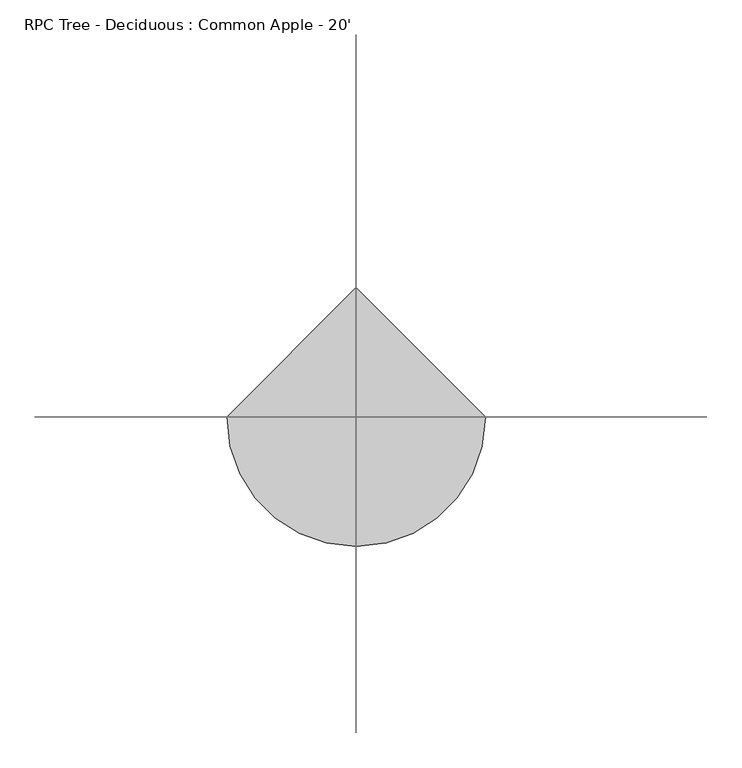
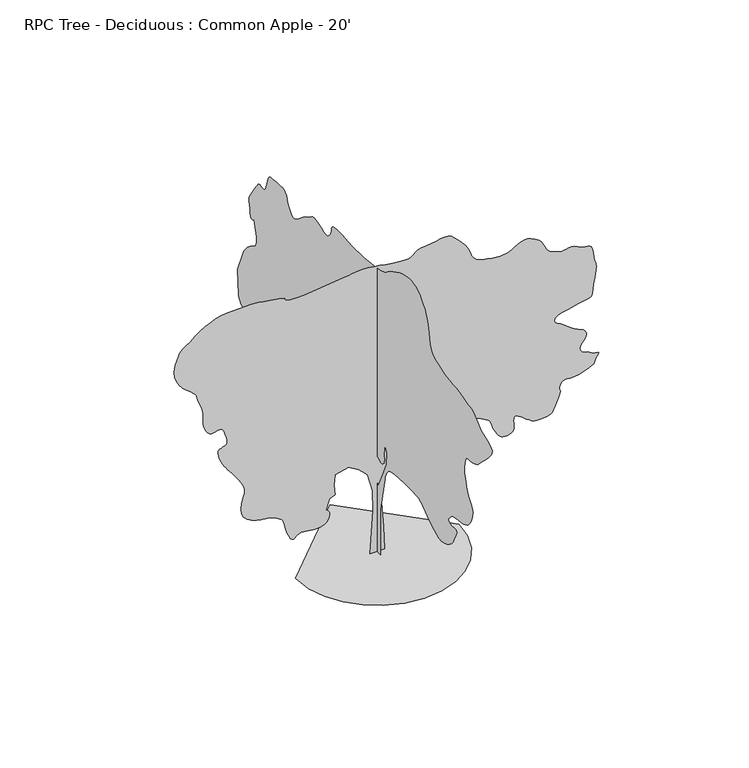
"""IFC4 building model written with IfcOpenShell, lengths in millimetres: geographic element geometry, RPC Tree - Deciduous : Common Apple - 20'."""

from ifc_helpers import new_model, si_unit, origin, place, context, project, spatial, triangles, source, transform, mapped, element, save


def rpc_tree_deciduous_common_apple_20_2cf08d23(model_context):
    return source(origin(), model_context, "Body", "Tessellation", [
        triangles([(-6.61e-05, -106.7031981, 0.0075972), (-6.25e-05, 141.1357166, 0.0075898), (-4.92e-05, 101.4814601, 465.9455781), (-3.19e-05, 131.2220957, 1031.0173004), (-1.83e-05, 230.3576144, 1437.4734501), (-8.7e-06, 398.8869896, 1675.3980263), (-1.1e-06, 587.2459139, 1834.016106), (2.7e-06, 765.6887283, 1873.6680462), (3.6e-06, 963.961219, 1804.2751888), (1.5e-06, 1023.4430534, 1705.1389435), (-4.1e-06, 904.4794573, 1576.2617809), (-8.5e-06, 944.1340136, 1407.7326782), (-1.46e-05, 1172.144878, 1090.4990622), (-1.49e-05, 1568.687534, 882.3128597), (-8.7e-06, 2143.6727863, 803.006436), (7.7e-06, 2490.6473923, 1179.7191977), (2.57e-05, 2847.5453751, 1606.0026981), (3.25e-05, 3402.6882339, 1556.4345028), (3.9e-05, 3600.9610153, 1675.3980263), (4.6e-05, 3591.0549339, 1913.3226025), (4.57e-05, 3412.6196045, 1992.6315697), (5.03e-05, 3283.7399712, 2210.7288677), (5.51e-05, 3591.0549339, 2220.6425068), (6.07e-05, 4205.6845688, 2101.6814541), (6.29e-05, 4275.3567696, 2137.8384041), (6.49e-05, 4342.3114037, 2174.2544952), (6.7e-05, 4403.9061905, 2211.1911942), (6.89e-05, 4457.4241447, 2248.9101128), (7.07e-05, 4500.1976967, 2287.6680668), (7.23e-05, 4529.5348595, 2327.7263775), (7.37e-05, 4542.7427742, 2369.3469475), (8.93e-05, 4572.4863075, 2874.9268433), (9.94e-05, 4403.9570595, 3301.215358), (0.0001002, 4386.5834106, 3334.8449913), (0.000101, 4360.9041641, 3374.6975006), (0.0001018, 4328.265168, 3418.5378479), (0.0001026, 4290.0887192, 3464.105706), (0.0001033, 4247.7471176, 3509.1651649), (0.0001039, 4202.636499, 3551.4561882), (0.0001043, 4156.1291634, 3588.718158), (0.0001045, 4111.323468, 3617.9027138), (0.0001046, 4070.8611122, 3640.1530998), (0.0001046, 4035.4281006, 3659.4571541), (0.0001048, 4005.7101471, 3679.8024239), (0.0001052, 3982.4182549, 3705.2026176), (0.000106, 3966.2384285, 3739.5941231), (0.0001073, 3957.8566727, 3786.9906487), (0.0001089, 3956.7898773, 3842.7945099), (0.0001107, 3961.4378494, 3899.6395866), (0.0001126, 3970.8614021, 3957.3738533), (0.0001145, 3984.0948967, 4015.7685448), (0.0001165, 4000.1982742, 4074.6966339), (0.0001185, 4018.2070587, 4133.9802246), (0.0001206, 4037.1553207, 4193.4417114), (0.0001203, 4062.5299347, 4172.9947037), (0.0001202, 4087.2188347, 4157.4244331), (0.0001204, 4110.5107269, 4151.5570587), (0.000121, 4131.7196068, 4160.2693176), (0.0001221, 4150.160051, 4188.3870781), (0.0001239, 4165.1460548, 4240.787368), (0.0001265, 4175.9410355, 4322.3213448), (0.000129, 4186.6092796, 4402.5600517), (0.0001308, 4198.1408432, 4455.5698975), (0.000132, 4205.3543564, 4492.9588943), (0.000133, 4202.9922913, 4526.3597626), (0.0001339, 4185.923275, 4567.406385), (0.0001352, 4148.8900703, 4627.7059021), (0.000137, 4086.736306, 4718.8666168), (0.0001389, 4019.8834099, 4816.9867905), (0.0001404, 3969.4896835, 4892.043837), (0.0001414, 3931.4405525, 4946.4759796), (0.0001421, 3901.5194138, 4982.6714447), (0.0001423, 3875.5858223, 5003.1184525), (0.0001421, 3849.5002052, 5010.2046478), (0.0001416, 3819.0709579, 5006.343837), (0.0001408, 3787.3208611, 4996.7176804), (0.0001401, 3759.4062859, 4987.6240494), (0.0001396, 3734.2601463, 4983.2045517), (0.0001394, 3710.841227, 4987.6240494), (0.0001396, 3688.1338921, 5005.0485672), (0.0001402, 3665.0704742, 5039.6435486), (0.0001416, 3640.6103394, 5095.574437), (0.0001432, 3619.2235634, 5160.9030075), (0.0001447, 3603.043737, 5219.9581238), (0.000146, 3587.5496246, 5271.4183548), (0.000147, 3568.2455704, 5313.8366959), (0.0001475, 3540.6103386, 5345.8661362), (0.0001475, 3500.1482735, 5366.109668), (0.0001469, 3442.3378487, 5373.1458664), (0.0001459, 3372.4368828, 5376.2445145), (0.0001451, 3300.6055115, 5383.3312912), (0.0001442, 3229.8412262, 5391.1034912), (0.0001434, 3163.0391991, 5396.2851517), (0.0001425, 3103.1713417, 5395.5485687), (0.0001414, 3053.2095657, 5385.642778), (0.0001402, 3016.0746231, 5363.2394943), (0.0001391, 2991.8429626, 5337.2044556), (0.0001382, 2976.4758774, 5316.3510773), (0.0001375, 2966.6462448, 5297.4283951), (0.0001368, 2959.0769394, 5277.1081238), (0.0001359, 2950.4664185, 5252.1148819), (0.0001348, 2937.5122673, 5219.1198029), (0.0001331, 2916.9382324, 5174.873085), (0.0001313, 2890.1666107, 5126.1051315), (0.0001296, 2860.6265533, 5083.2042618), (0.000128, 2827.9619774, 5048.4569641), (0.0001268, 2791.8432518, 5024.124147), (0.0001258, 2751.8890045, 5012.4399765), (0.0001253, 2707.794603, 5015.6909409), (0.0001252, 2659.1789658, 5036.0873703), (0.0001254, 2610.791803, 5068.0662323), (0.0001258, 2565.8846603, 5103.6768494), (0.0001263, 2521.8332794, 5141.7006912), (0.0001267, 2476.0523529, 5180.9436447), (0.0001272, 2425.9356445, 5220.212178), (0.0001274, 2368.8821503, 5258.2360199), (0.0001275, 2302.2908661, 5293.846637), (0.0001276, 2240.2945049, 5328.4671982), (0.0001279, 2193.5584042, 5362.0459625), (0.0001282, 2154.2798424, 5391.129071), (0.0001282, 2114.6558075, 5412.2365036), (0.0001278, 2066.8783459, 5421.8882401), (0.0001267, 2003.1496777, 5416.6304214), (0.0001247, 1915.6618492, 5392.9830276), (0.0001224, 1826.1497257, 5361.2837997), (0.0001207, 1757.9710384, 5335.9853439), (0.0001194, 1705.7434124, 5319.8816757), (0.0001187, 1664.0950825, 5315.7418121), (0.0001184, 1627.6484699, 5326.358606), (0.0001187, 1591.0293388, 5354.4766571), (0.0001195, 1548.8602558, 5402.8893997), (0.0001207, 1514.8419834, 5459.7853455), (0.000122, 1498.8602554, 5510.7630478), (0.0001232, 1489.8128426, 5554.806871), (0.0001241, 1476.6047825, 5590.874437), (0.0001244, 1448.1338459, 5617.9256927), (0.0001241, 1393.3079773, 5634.9182602), (0.0001229, 1301.0220406, 5640.8109238), (0.0001214, 1201.3955635, 5639.6935501), (0.0001202, 1126.7398006, 5636.6454803), (0.0001192, 1069.2519579, 5632.2259827), (0.0001184, 1021.1290958, 5626.9425842), (0.0001175, 974.5682751, 5621.3039749), (0.0001165, 921.7642307, 5615.8426804), (0.0001154, 854.9113346, 5611.0679718), (0.0001143, 784.7082069, 5608.019902), (0.0001133, 723.0014357, 5607.2071609), (0.0001125, 663.7228592, 5608.4768509), (0.0001116, 600.8019178, 5611.6516571), (0.0001107, 528.1680156, 5616.5792633), (0.0001096, 439.7556433, 5623.0567749), (0.0001082, 329.4941322, 5630.9051331), (0.0001067, 206.9466705, 5641.7254028), (0.0001053, 88.3885184, 5656.6861176), (0.0001042, -22.1921751, 5675.1262711), (0.0001034, -120.8075788, 5696.3354416), (0.0001029, -203.4686488, 5719.6276245), (0.0001027, -266.1871316, 5744.3162338), (0.0001028, -304.9729546, 5769.6908478), (0.0001032, -347.9523442, 5804.4381454), (0.0001036, -420.583703, 5853.4089935), (0.0001039, -514.8939712, 5910.1532043), (0.000104, -622.9024584, 5968.31884), (0.0001039, -736.6335978, 6021.4301331), (0.0001035, -848.1092062, 6063.1118912), (0.0001027, -949.3562239, 6086.9371811), (0.0001016, -1039.2697763, 6095.8017563), (0.0001004, -1122.4243664, 6096.0046509), (9.9e-05, -1199.3330441, 6086.1494385), (9.73e-05, -1270.5191059, 6064.8391113), (9.53e-05, -1336.5033051, 6030.7016602), (9.29e-05, -1397.8062492, 5982.3650757), (9.01e-05, -1454.9462208, 5918.407933), (8.77e-05, -1502.3755932, 5861.1056168), (8.62e-05, -1536.9730453, 5825.4944183), (8.5e-05, -1562.8963177, 5799.256485), (8.38e-05, -1584.313615, 5770.0716385), (8.22e-05, -1605.3828232, 5725.6220261), (7.96e-05, -1630.2698215, 5653.5874695), (7.58e-05, -1663.1323505, 5541.6751144), (7.16e-05, -1693.8258259, 5415.6147858), (6.81e-05, -1715.6747829, 5307.5626602), (6.5e-05, -1738.0446384, 5214.9799393), (6.21e-05, -1770.3000824, 5135.1981812), (5.93e-05, -1821.8062408, 5065.6530075), (5.62e-05, -1901.9230076, 5003.7532974), (5.28e-05, -2020.0178341, 4946.8823502), (4.95e-05, -2152.913356, 4902.7117905), (4.69e-05, -2273.494804, 4876.3974083), (4.48e-05, -2385.2295536, 4861.5384315), (4.29e-05, -2491.5921021, 4851.7340881), (4.1e-05, -2596.0345642, 4840.5071571), (3.89e-05, -2702.0542557, 4821.482737), (3.62e-05, -2813.1030006, 4788.2594742), (3.39e-05, -2912.3155495, 4758.5159409), (3.24e-05, -2986.585144, 4746.9843773), (3.14e-05, -3044.8780975, 4742.742485), (3.04e-05, -3096.2371719, 4734.8432579), (2.89e-05, -3149.6786774, 4712.3896866), (2.66e-05, -3214.2200867, 4664.4344742), (2.28e-05, -3298.878582, 4580.0809021), (1.85e-05, -3408.6320572, 4492.8062874), (1.5e-05, -3530.0185432, 4434.3354378), (1.2e-05, -3644.3188339, 4390.95233), (9.4e-06, -3732.7616913, 4348.9659393), (7.2e-06, -3776.6273277, 4294.6608238), (5.1e-06, -3757.196537, 4214.3459587), (3e-06, -3655.7486595, 4094.3056114), (1.1e-06, -3529.027906, 3968.7786804), (-3e-07, -3439.3912262, 3876.7287758), (-1.3e-06, -3376.6531952, 3811.5525215), (-1.9e-06, -3330.5522301, 3766.670668), (-2.3e-06, -3290.852037, 3735.479258), (-2.3e-06, -3247.3671913, 3711.4002045), (-2.2e-06, -3189.8108208, 3687.854258), (-1.7e-06, -3124.3802216, 3671.1919029), (-1e-06, -3064.487075, 3666.3404549), (-2e-07, -3010.8420937, 3664.4356293), (2e-07, -2964.1568619, 3656.6378494), (2e-07, -2925.0662247, 3634.0825401), (-8e-07, -2894.3070557, 3587.9559952), (-2.8e-06, -2872.5897766, 3509.3939301), (-5.1e-06, -2860.8041588, 3423.8465355), (-7.1e-06, -2858.3659355, 3357.9081184), (-8.8e-06, -2863.7507813, 3304.4410332), (-1.04e-05, -2875.358503, 3256.3335045), (-1.21e-05, -2891.6653564, 3206.498465), (-1.41e-05, -2911.070858, 3147.8244301), (-1.67e-05, -2932.0768433, 3073.199334), (-1.95e-05, -2961.2613991, 2993.8242371), (-2.22e-05, -3001.7234642, 2923.6186386), (-2.47e-05, -3046.5291595, 2859.6612053), (-2.72e-05, -3088.7187355, 2798.9806068), (-2.95e-05, -3121.3830208, 2738.6555099), (-3.16e-05, -3137.5628471, 2675.7398735), (-3.35e-05, -3130.349334, 2607.2612045), (-3.52e-05, -3109.3942177, 2540.281572), (-3.66e-05, -3087.7280983, 2482.819091), (-3.77e-05, -3063.4964378, 2433.5098915), (-3.85e-05, -3034.7182526, 2390.964814), (-3.91e-05, -2999.5645844, 2353.7970245), (-3.94e-05, -2956.0544495, 2320.6169277), (-3.96e-05, -2902.3333099, 2290.0378349), (-3.93e-05, -2836.3948929, 2266.2507694), (-3.86e-05, -2760.9314758, 2251.4832115), (-3.77e-05, -2680.9721123, 2241.3942924), (-3.68e-05, -2601.4955681, 2231.6559334), (-3.61e-05, -2527.6041481, 2217.9272655), (-3.58e-05, -2464.279525, 2195.8749779), (-3.62e-05, -2416.56049, 2161.1632885), (-3.68e-05, -2383.2356346, 2123.2410393), (-3.73e-05, -2359.9691769, 2093.2995529), (-3.79e-05, -2347.1065899, 2069.598674), (-3.84e-05, -2344.9984337, 2050.4090023), (-3.9e-05, -2353.9875652, 2033.9929985), (-3.98e-05, -2374.4217831, 2018.6158848), (-4.07e-05, -2406.646851, 2002.5452087), (-4.16e-05, -2449.8269188, 1993.9041664), (-4.23e-05, -2498.3841293, 1996.5330757), (-4.28e-05, -2545.5646797, 2002.2862129), (-4.34e-05, -2584.5791588, 2003.0075352), (-4.41e-05, -2608.6837921, 1990.5513187), (-4.52e-05, -2611.0967262, 1956.7642822), (-4.66e-05, -2585.0869766, 1893.4953243), (-4.83e-05, -2549.9080193, 1821.1814243), (-4.96e-05, -2524.6272949, 1762.91376), (-5.07e-05, -2502.1126808, 1714.5318295), (-5.16e-05, -2475.2625755, 1671.8725147), (-5.23e-05, -2436.9668026, 1630.7726978), (-5.27e-05, -2380.1140228, 1587.0720222), (-5.3e-05, -2297.5969666, 1536.6072247), (-5.28e-05, -2203.8378639, 1496.8968578), (-5.19e-05, -2116.842738, 1484.7582092), (-5.03e-05, -2034.8743401, 1494.9892708), (-4.83e-05, -1956.2028339, 1522.3883251), (-4.6e-05, -1879.090971, 1561.7532188), (-4.35e-05, -1801.803828, 1607.8822346), (-4.09e-05, -1722.6115688, 1655.5707481), (-3.83e-05, -1647.9584221, 1703.6352562), (-3.59e-05, -1583.013113, 1752.3931812), (-3.37e-05, -1524.1383636, 1798.8980461), (-3.16e-05, -1467.6919544, 1840.2010483), (-2.97e-05, -1410.0313751, 1873.3506237), (-2.82e-05, -1347.5167316, 1895.4053822), (-2.69e-05, -1276.503479, 1903.4089634), (-2.54e-05, -1177.6846561, 1904.2776604), (-2.33e-05, -1044.3574018, 1905.4916851), (-2.11e-05, -891.7820492, 1904.9710773), (-1.89e-05, -735.2163151, 1900.6352955), (-1.7e-05, -589.9230761, 1890.4040886), (-1.58e-05, -471.1627742, 1872.1948803), (-1.55e-05, -394.1956335, 1843.9297451), (-1.6e-05, -348.7041879, 1805.3140789), (-1.68e-05, -313.0958962, 1758.377409), (-1.8e-05, -285.7248199, 1704.5039532), (-1.95e-05, -264.9450744, 1645.0805454), (-2.11e-05, -249.1058704, 1581.494165), (-2.29e-05, -236.5620685, 1515.1341167), (-2.48e-05, -225.6659676, 1447.3870892), (-3.91e-05, -116.6168281, 912.0537769), (-2.05e-05, -27.3946828, 1318.5099266), (-1.32e-05, -176.0980811, 1635.74347), (-6.6e-06, -304.975498, 1923.2362415), (2e-07, -324.8002327, 2161.1632885), (4.8e-06, -255.4073572, 2280.1241959), (-4e-07, -225.6657133, 2091.767815), (-1.7e-06, -231.7353101, 2049.4539734), (-3e-06, -235.984215, 2008.1814926), (-4.2e-06, -236.5910275, 1968.9892628), (-5.2e-06, -231.7353101, 1932.9186447), (-6e-06, -219.5961346, 1901.0111446), (-6.5e-06, -198.3530817, 1874.3056526), (-6.6e-06, -166.1844602, 1853.8433842), (-6.2e-06, -129.2182845, 1848.5829494), (-5.3e-06, -95.0268123, 1860.3152275), (-4.3e-06, -63.9562343, 1879.3348515), (-3.4e-06, -36.354542, 1895.9235191), (-2.9e-06, -12.5678035, 1900.3761543), (-3.1e-06, 7.0569383, 1882.9772163), (-4.4e-06, 22.1729471, 1834.016106), (-6.1e-06, 32.8958209, 1768.9260384), (-7.8e-06, 39.9768386, 1709.0403042), (-9.4e-06, 44.0233167, 1653.4904972), (-1.1e-05, 45.6418044, 1601.4077751), (-1.24e-05, 45.4396183, 1551.9260571), (-1.39e-05, 44.0233167, 1504.1789715), (-1.53e-05, 41.9999482, 1457.3007282), (139.590126, 0.0003305, 0.0), (-135.4471285, 0.0003387, 0.0), (-74.3278259, 0.000241, 845.4879272), (-84.5142454, 0.0002472, 1242.76455), (-186.3807747, 0.0002013, 1599.294532), (-339.1791879, 0.0002082, 1752.0933449), (-542.9102117, 0.000216, 1874.3335579), (-797.5758808, 0.0002227, 1813.2134514), (-817.9492012, 0.0002203, 1609.4824276), (-797.5758808, 0.0002168, 1415.9368286), (-899.4426281, 0.0002191, 1365.0021469), (-970.7481594, 0.0002183, 1171.4565479), (-951.3247084, 0.0002718, 1158.1240768), (-933.2373676, 0.000271, 1143.3616058), (-917.8246456, 0.0002703, 1125.7517796), (-906.4200365, 0.0002696, 1103.8645981), (-900.3621214, 0.000269, 1076.2750757), (-900.9870106, 0.0002686, 1041.555756), (-909.6280529, 0.0002682, 998.2868128), (-928.5764603, 0.0002681, 955.1042742), (-957.6798437, 0.0002684, 921.0098436), (-994.6267164, 0.0002692, 895.1144766), (-1037.0955631, 0.0002701, 876.5217161), (-1082.7698101, 0.0002713, 864.3449158), (-1129.3382612, 0.0002726, 857.6926329), (-1174.4791832, 0.0002739, 855.6733521), (-1218.6700905, 0.0002753, 858.4063974), (-1263.5747623, 0.0002767, 865.0586803), (-1308.6573303, 0.0002782, 873.3161705), (-1353.3816353, 0.0002796, 880.857498), (-1397.217041, 0.000281, 885.3710306), (-1439.6273884, 0.0002823, 884.5404854), (-1480.0769543, 0.0002833, 876.0466724), (-1514.854628, 0.0002841, 857.900905), (-1542.5051205, 0.0002846, 834.4084436), (-1565.8782578, 0.000285, 812.6990856), (-1587.8238659, 0.0002854, 799.9000122), (-1611.1970032, 0.0002862, 803.1359339), (-1638.8473503, 0.0002874, 829.5392641), (-1673.6225533, 0.000235, 886.2346407), (-1706.6171963, 0.0002371, 959.4984827), (-1729.2790398, 0.0002388, 1029.5593225), (-1744.988982, 0.0002402, 1094.4487484), (-1757.1353336, 0.0002415, 1152.2135365), (-1769.1037891, 0.0002426, 1200.8900711), (-1784.2803337, 0.0002436, 1238.5177162), (-1806.0481911, 0.0002446, 1263.1378704), (-1833.1626698, 0.0002457, 1282.7670502), (-1863.3073414, 0.0002469, 1305.4288937), (-1898.2629112, 0.0002483, 1329.1576778), (-1939.8122646, 0.0002499, 1351.9948013), (-1989.7334908, 0.0002517, 1371.9820988), (-2049.8147072, 0.0002537, 1387.1586433), (-2121.8338577, 0.000256, 1395.5635082), (-2205.4938675, 0.0002044, 1404.6210949), (-2294.67854, 0.0002073, 1424.3695988), (-2382.4381542, 0.0002104, 1456.7724174), (-2461.8232796, 0.0002135, 1503.7853909), (-2525.8821602, 0.0002163, 1567.3691551), (-2567.6627495, 0.0002188, 1649.4849277), (-2580.2355286, 0.0002207, 1752.0933449), (-2568.9835991, 0.0002218, 1851.4048702), (-2548.8159348, 0.0002224, 1927.9097935), (-2527.0379036, 0.0002227, 1989.979842), (-2510.9723145, 0.0001688, 2045.9893593), (-2507.9117455, 0.0001695, 2104.3180664), (-2525.1659248, 0.0001711, 2173.3375454), (-2570.0503944, 0.0001737, 2261.4222851), (-2629.7912247, 0.0001769, 2355.7756828), (-2686.3316689, 0.0001798, 2438.7243988), (-2738.9604332, 0.0001825, 2511.3356644), (-2786.9665146, 0.0001849, 2574.6730774), (-2829.6130394, 0.0001327, 2629.841803), (-2866.1890045, 0.0001345, 2677.8478844), (-2896.008696, 0.000136, 2719.8086952), (-2924.6092758, 0.0001376, 2767.4084061), (-2955.1652596, 0.0001394, 2827.2762634), (-2983.4100471, 0.0001412, 2893.0114952), (-3005.0764572, 0.0001428, 2958.2389091), (-3015.8461487, 0.000144, 3016.5062828), (-3011.4772293, 0.0001446, 3061.4137161), (-2987.7028084, 0.0001442, 3086.5342758), (-2951.4823448, 0.0001433, 3098.8532913), (-2915.109565, 0.0001425, 3111.5533882), (-2882.1147766, 0.0001417, 3127.4282913), (-2856.0800285, 0.0001413, 3149.3740448), (-2840.5350471, 0.0001413, 3180.2349518), (-2839.0871704, 0.0001418, 3222.8561874), (-2855.2669968, 0.0001432, 3280.0823456), (-2877.0348541, 9.05e-05, 3338.9342766), (-2892.2240433, 9.16e-05, 3385.5177704), (-2904.1875572, 9.25e-05, 3421.2048363), (-2916.3286766, 9.32e-05, 3447.4686401), (-2932.0259743, 9.4e-05, 3465.705899), (-2954.70802, 9.48e-05, 3477.3389099), (-2987.7028084, 9.59e-05, 3483.8161308), (-3026.4123642, 9.7e-05, 3481.8857254), (-3064.2583099, 9.8e-05, 3472.1066711), (-3101.5455688, 9.9e-05, 3461.6419029), (-3138.6805115, 0.0001, 3457.552327), (-3175.9930595, 0.0001013, 3467.026458), (-3213.8137161, 0.0001029, 3497.1763618), (-3252.5488518, 0.0001049, 3555.1138138), (-3281.1747208, 0.0001068, 3626.7419998), (-3293.239682, 0.0001082, 3695.3474052), (-3295.8558014, 0.0001093, 3764.1307068), (-3296.1351448, 0.0001104, 3836.3175797), (-3301.2406471, 5.74e-05, 3915.0575409), (-3318.2840836, 5.93e-05, 4003.6274254), (-3354.4028091, 6.19e-05, 4105.2020393), (-3391.2836975, 6.43e-05, 4197.0231789), (-3411.2481766, 6.59e-05, 4259.8120789), (-3422.2972115, 6.68e-05, 4301.925206), (-3432.4570564, 6.76e-05, 4331.7448975), (-3449.7545471, 6.85e-05, 4357.6276199), (-3482.1650688, 6.99e-05, 4387.9804184), (-3537.7657448, 7.22e-05, 4431.1606316), (-3609.6985634, 2.09e-05, 4488.5646858), (-3681.631382, 2.41e-05, 4556.1285851), (-3747.3157448, 2.72e-05, 4634.0305161), (-3800.5287758, 3.01e-05, 4722.4480843), (-3835.047599, 3.26e-05, 4821.5588951), (-3844.6231773, 3.45e-05, 4931.5152649), (-3822.9823471, 3.57e-05, 5052.5468307), (-3789.555899, -1.8e-05, 5157.9310959), (-3763.7749146, -1.77e-05, 5228.187854), (-3739.5941231, -1.77e-05, 5274.3902664), (-3710.9682541, -1.81e-05, 5307.5882401), (-3671.8270386, -1.88e-05, 5338.8555176), (-3616.1246246, -1.98e-05, 5379.1652664), (-3537.7657448, -2.13e-05, 5439.6429703), (-3445.4364967, -2.3e-05, 5511.6775269), (-3351.6849518, -2.48e-05, 5578.225209), (-3256.3079247, -2.67e-05, 5637.4326416), (-3159.1783882, -2.89e-05, 5687.5726044), (-3060.0675774, -3.12e-05, 5726.8155579), (-2958.8228851, -3.39e-05, 5753.4348633), (-2855.2669968, -3.68e-05, 5765.6015625), (-2376.4970924, -5.09e-05, 5775.7869873), (-2309.7356152, -5.29e-05, 5773.1197083), (-2232.8167637, -5.53e-05, 5765.6521408), (-2147.4320045, -3.8e-06, 5754.1458664), (-2055.2781818, -6.7e-06, 5739.4392059), (-1958.0469074, -9.9e-06, 5722.3449005), (-1857.4273224, -1.32e-05, 5703.6251129), (-1755.1159801, -1.65e-05, 5684.1181641), (-1751.9080364, -1.69e-05, 5664.6617935), (-1742.5530842, -1.75e-05, 5646.3739563), (-1720.9022255, -1.83e-05, 5630.3970245), (-1680.8107773, -1.97e-05, 5617.9001129), (-1616.1270802, -2.18e-05, 5610.0261749), (-1520.7042709, -2.46e-05, 5607.9437439), (-1388.3981026, -2.85e-05, 5612.8201904), (-614.2181774, -5.02e-05, 5704.4890137), (-538.3076946, -5.24e-05, 5711.4996323), (-472.1990845, 1e-07, 5721.8879517), (-409.4762778, -1.6e-06, 5732.8355392), (-343.7232419, -3.5e-06, 5741.4460602), (-268.5264692, -5.7e-06, 5744.8749207), (-177.4707081, -8.5e-06, 5740.3031067), (-64.1414019, -1.21e-05, 5724.8598633), (54.7118994, -1.59e-05, 5704.3111176), (159.4882483, -1.93e-05, 5686.4296509), (252.3260954, -2.23e-05, 5671.4183578), (335.3640864, -2.49e-05, 5659.4039749), (410.7386644, -2.73e-05, 5650.6155579), (480.5886887, -2.95e-05, 5645.205423), (547.0529457, -3.15e-05, 5643.3764648), (603.2428662, -3.3e-05, 5651.8346695), (646.0698669, -3.4e-05, 5673.6531052), (683.3697704, -3.47e-05, 5703.4983765), (722.9887184, -3.54e-05, 5736.0359253), (772.7625698, -3.64e-05, 5765.8806152), (840.5349592, -3.81e-05, 5787.6996323), (934.1441437, -4.07e-05, 5796.1828354), (1035.6832947, -4.37e-05, 5802.989978), (1124.0372766, -4.61e-05, 5818.3826431), (1202.2337391, -4.82e-05, 5834.6642075), (1273.3004768, -5.01e-05, 5844.1636276), (1340.2726971, -5.22e-05, 5839.2360214), (1406.173035, -5.46e-05, 5812.2103455), (1474.0342999, -3.2e-06, 5755.4161377), (1539.0152172, -6.2e-06, 5686.9627579), (1594.7301304, -8.7e-06, 5628.1366974), (1641.8903332, -1.09e-05, 5576.0666199), (1681.2120609, -1.28e-05, 5527.9335114), (1713.4041367, -1.44e-05, 5480.8671982), (1739.182505, -1.59e-05, 5431.9975067), (1759.2587505, -1.73e-05, 5378.5304214), (1777.3156425, -1.87e-05, 5324.8604416), (1798.9361252, -2e-05, 5277.2604401), (1827.6839344, -2.15e-05, 5235.5281036), (1867.1225155, 3.1e-05, 5199.4855362), (1920.8180752, 2.9e-05, 5169.0060013), (1992.3318787, 2.65e-05, 5143.8342819), (2085.229842, 2.34e-05, 5123.844223), (2181.6306438, 2.03e-05, 5109.4171967), (2262.7075264, 1.78e-05, 5100.6799393), (2330.5991673, 1.57e-05, 5097.123761), (2387.4419186, 1.4e-05, 5098.1905563), (2435.3767834, 1.27e-05, 5103.3722168), (2476.5374977, 1.16e-05, 5112.0844757), (2513.0678261, 1.07e-05, 5123.844223), (2552.2195061, 9.8e-06, 5144.4947067), (2599.1840813, 8.9e-06, 5175.4829315), (2653.1336952, 7.8e-06, 5209.6459625), (2713.1032906, 6.4e-06, 5239.9226028), (2778.2795448, 4.8e-06, 5259.1249191), (2847.697982, 2.7e-06, 5260.1661346), (2920.5196999, 2e-07, 5235.9094757), (2984.2992371, -2.2e-06, 5202.1528152), (3030.2478859, -4e-06, 5176.5747253), (3062.9883293, -5.3e-06, 5154.908606), (3087.1947006, -6.3e-06, 5132.9122742), (3107.4893921, -7.3e-06, 5106.2679703), (3128.4697975, -8.5e-06, 5070.73293), (3154.8094688, -1e-05, 5021.9905563), (3182.8510712, 4.27e-05, 4971.0890121), (3208.2256851, 4.13e-05, 4930.3473129), (3234.4639091, 4e-05, 4897.4289734), (3265.1724998, 3.87e-05, 4870.0475052), (3303.9076355, 3.72e-05, 4845.8667137), (3354.2252037, 3.53e-05, 4822.6004013), (3419.6808014, 3.3e-05, 4797.8859215), (3486.0258797, 3.08e-05, 4782.8237595), (3540.0769409, 2.92e-05, 4784.7032959), (3586.9909378, 2.8e-05, 4795.4729874), (3631.9489494, 2.68e-05, 4807.1571579), (3680.1326363, 2.55e-05, 4811.7036827), (3736.6730804, 2.36e-05, 4801.0863075), (3806.7519424, 2.1e-05, 4767.3299377), (3879.2181587, 1.84e-05, 4732.9890106), (3939.9240463, 1.63e-05, 4718.4346664), (3989.5811897, 1.48e-05, 4712.2626595), (4028.9003014, 1.35e-05, 4703.0678719), (4058.6185455, 1.22e-05, 4679.4204781), (4079.3957657, 6.51e-05, 4629.9412308), (4091.9941246, 6.34e-05, 4543.2253029), (4103.8306114, 6.18e-05, 4454.6301292), (4119.4261711, 6.04e-05, 4397.0481789), (4135.0217308, 5.94e-05, 4355.3161331), (4146.8835068, 5.84e-05, 4314.2950905), (4151.2268463, 5.74e-05, 4258.8467308), (4144.3688347, 5.64e-05, 4173.8330246), (4122.550399, 5.51e-05, 4044.0642014), (4100.096537, 0.000108, 3908.7329269), (4088.8698967, 0.0001069, 3812.0603394), (4081.3767494, 0.0001061, 3746.5791618), (4070.1501091, 0.0001058, 3704.7962471), (4047.6965378, 0.0001061, 3679.2184479), (4006.548468, 0.0001071, 3662.4034859), (3939.1874634, 0.0001089, 3646.8079262), (3844.4708611, 0.0001114, 3628.5706673), (3734.0822502, 0.0001144, 3608.1998177), (3619.7822502, 0.0001175, 3584.781189), (3513.3053192, 0.0001202, 3557.4761696), (3426.4373657, 0.0001224, 3525.3449913), (3370.9384277, 0.0001234, 3487.4990456), (3358.5429634, 0.0001231, 3443.0744316), (3371.5224037, 0.0001222, 3405.6092766), (3386.2799332, 0.0001214, 3384.1972115), (3405.8633308, 0.0001207, 3371.1669022), (3433.2700882, 0.0001197, 3358.8478867), (3471.5476936, 0.0001182, 3339.5694122), (3523.7447983, 0.0001162, 3305.6857246), (3592.8327324, 0.0001133, 3249.5260712), (3669.2870773, 0.0001101, 3189.9884262), (3740.381575, 0.0001074, 3147.3671906), (3804.5419029, 0.000105, 3116.150782), (3860.1425789, 0.0001572, 3090.8014572), (3905.55783, 0.0001555, 3065.8332138), (3939.2383324, 0.000154, 3035.6833099), (3959.558313, 0.0001528, 2994.8654526), (3960.2948959, 0.0001521, 2946.884951), (3941.8038734, 0.0001519, 2899.2852402), (3912.2635254, 0.0001521, 2852.3968231), (3879.8530037, 0.0001524, 2806.5752014), (3852.8020386, 0.0001525, 2762.1758766), (3839.2892006, 0.0001523, 2719.554641), (3847.5189308, 0.0001514, 2679.0672867), (3870.582058, 0.0001503, 2647.1645828), (3896.1598572, 0.0001492, 2627.2256836), (3924.2270393, 0.0001482, 2614.9319572), (3954.7830231, 0.0001472, 2606.0168037), (3987.8286804, 0.000146, 2596.2121696), (4023.3887192, 0.0001447, 2581.2517456), (4061.4378502, 0.0001432, 2556.842189), (4100.7569618, 0.0001417, 2534.5891869), (4137.7648773, 0.0001405, 2524.8203064), (4168.8798386, 0.0001395, 2521.2847664), (4190.5462486, 0.0001388, 2517.7515518), (4199.2329277, 0.0001384, 2507.9803459), (4191.3334099, 0.0001926, 2485.7375175), (4163.2918076, 0.0001928, 2444.7824593), (4135.3263634, 0.0001929, 2399.7888393), (4122.8550316, 0.0001928, 2366.7332989), (4115.1842789, 0.0001927, 2341.3408081), (4101.6461517, 0.0001927, 2319.3343025), (4071.521537, 0.0001933, 2296.4387524), (4014.1430626, 0.0001946, 2268.3717155), (3918.8166138, 0.0001969, 2230.8633945), (3811.1205711, 0.0001996, 2200.6297749), (3722.1443161, 0.0002021, 2191.0666958), (3649.3987564, 0.0002043, 2192.9081532), (3590.3436401, 0.0002062, 2196.8884335), (3542.540744, 0.0002075, 2193.7413872), (3503.4501068, 0.0002084, 2174.1985394), (3470.6079254, 0.0002087, 2128.9966473), (3451.2532928, 0.0002086, 2081.7474964), (3449.1702805, 0.0002083, 2055.3443115), (3456.7142967, 0.0002078, 2039.4564732), (3466.2137169, 0.0002073, 2023.7466763), (3470.0236588, 0.0002068, 1997.8792145), (3460.4480804, 0.0002064, 1951.5191082), (3429.8662262, 0.0002061, 1874.3335579), (3393.2393921, 0.0002059, 1787.376511), (3366.4171921, 0.0002057, 1717.5239433), (3342.9982727, 0.0002056, 1663.1755165), (3316.5315742, 0.0002058, 1622.7259506), (3280.6157433, 0.0002064, 1594.5725819), (3228.850589, 0.0002077, 1577.1101303), (3154.8094688, 0.0002098, 1568.7357868), (3080.6413216, 0.0002119, 1565.2609989), (3027.8349518, 0.0002135, 1564.6361824), (2989.0998161, 0.0002147, 1568.469088), (2957.146534, 0.0002158, 1578.3572926), (2924.6598541, 0.000217, 1595.9086922), (2884.3248161, 0.0002186, 1622.7259506), (2828.8511673, 0.0002209, 1660.4146385), (2768.830703, 0.0002233, 1702.4363468), (2719.1482704, 0.0002253, 1739.6499184), (2678.9146797, 0.000227, 1769.7336926), (2647.2154518, 0.0002282, 1790.3763279), (2623.1869766, 0.0002291, 1799.2561638), (2605.9403549, 0.0002295, 1794.0567719), (2594.5613983, 0.0002295, 1772.4668106), (2588.1350464, 0.0002293, 1744.7273701), (2585.6459541, 0.000229, 1721.445797), (2586.0014557, 0.0002287, 1700.833683), (2588.1350464, 0.0002283, 1681.1130844), (2591.00522, 0.0002279, 1660.5034412), (2593.494603, 0.0002275, 1637.219252), (2594.5613983, 0.0002271, 1609.4824276), (2593.1135216, 0.0002267, 1579.0989624), (2587.906572, 0.0002264, 1549.7873795), (2577.7211472, 0.0002263, 1522.6143288), (2561.2872665, 0.0002264, 1498.6468964), (2537.3884346, 0.0002268, 1478.9568192), (2504.7494385, 0.0002276, 1464.6108925), (2462.1331444, 0.0002288, 1456.6836147), (2418.7144283, 0.00023, 1454.9893867), (2382.9562912, 0.0002312, 1459.35569), (2352.5447754, 0.0002322, 1470.8491745), (2325.1635979, 0.0002333, 1490.5392517), (2298.4935688, 0.0002346, 1519.4951878), (2270.2207306, 0.000236, 1558.7865395), (2238.0288002, 0.0002377, 1609.4824276), (2208.2396301, 0.0002394, 1664.8392231), (2186.8274197, 0.0001866, 1716.8127949), (2170.9397266, 0.0001878, 1764.5088661), (2157.7241089, 0.0001888, 1807.0362122), (2144.3307404, 0.0001897, 1843.5054977), (2127.9070335, 0.0001907, 1873.0254982), (2105.6033077, 0.0001917, 1894.7068783), (2074.6583942, 0.0001929, 1913.6528149), (2035.1589157, 0.0001944, 1935.2732975), (1988.5319653, 0.0001961, 1959.1214058), (1936.2028919, 0.0001981, 1984.7525448), (1879.5964634, 0.0002001, 2011.717178), (1820.1400635, 0.0002023, 2039.5759426), (1759.2587505, 0.0002046, 2067.8791569), (1412.9141933, 0.0002149, 2067.8791569), (1219.3685944, 0.0002173, 1843.7721966), (1214.8270838, 0.000217, 1813.2134514), (1209.2136909, 0.0002167, 1782.6522354), (1201.4616205, 0.0002165, 1752.0933449), (1190.5040045, 0.0002164, 1721.5345997), (1175.2665625, 0.0002164, 1690.9733837), (1154.6874407, 0.0002165, 1660.4146385), (1127.6898153, 0.0002169, 1629.855748), (1103.6638836, 0.0002172, 1604.0163368), (1088.903956, 0.0002174, 1586.5538853), (1077.7076191, 0.0002175, 1575.8629681), (1064.3726046, 0.0002179, 1570.3384506), (1043.1966442, 0.0002185, 1568.3775238), (1008.4798679, 0.0002195, 1568.3775238), (954.5175367, 0.0002211, 1568.7357868), (886.9839409, 0.0002232, 1571.6161343), (817.1339167, 0.0002254, 1579.3072346), (747.6394667, 0.0002276, 1590.3841747), (681.1726662, 0.0002298, 1603.4220417), (620.41075, 0.0002318, 1616.9957771), (568.0206702, 0.0002335, 1629.6755264), (526.6821324, 0.0002349, 1640.0411728), (491.1627162, 0.0002361, 1650.5543392), (454.5739975, 0.0002374, 1664.275304), (417.0937271, 0.0002388, 1680.6684895), (378.9022719, 0.0002402, 1699.2003525), (340.1748393, 0.0001874, 1719.3350246), (301.0918324, 0.0001889, 1740.5414337), (261.828495, 0.0001904, 1762.2813858), (78.4708189, 0.0002443, 1375.1901878), (68.2843994, 0.0002402, 1079.7776962), (119.217278, 0.0002837, 458.3966929), (-1547.0796959, 1.1e-06, 0.0099807), (-1506.1805935, -354.4877738, 0.0099913), (-1389.6986046, -680.02964, 0.010001), (-1206.9607035, -967.2962626, 0.0100095), (-967.2962626, -1206.9607035, 0.0100167), (-680.02964, -1389.6986046, 0.0100221), (-354.4877738, -1506.1805935, 0.0100256), (6.76e-05, -1547.0796959, 0.0100268), (354.4877738, -1506.1805935, 0.0100256), (680.02964, -1389.6986046, 0.0100221), (967.2962626, -1206.9607035, 0.0100167), (1206.9607035, -967.2962626, 0.0100095), (1389.6986046, -680.02964, 0.010001), (1506.1805935, -354.4877738, 0.0099913), (1547.0796959, 0.0001258, 0.0099807), (-0.0002029, 1547.0796959, 0.0099346)], [[300, 1, 301], [299, 300, 301], [299, 301, 302], [298, 299, 302], [297, 298, 302], [296, 297, 302], [296, 302, 303], [295, 296, 303], [294, 295, 303], [293, 294, 303], [292, 293, 303], [1, 2, 3], [301, 1, 3], [301, 3, 4], [301, 4, 5], [327, 301, 5], [326, 327, 5], [326, 5, 6], [325, 326, 6], [324, 325, 6], [323, 324, 6], [322, 323, 6], [321, 322, 6], [320, 321, 6], [19, 20, 21], [18, 19, 21], [17, 18, 21], [17, 21, 22], [320, 6, 7], [319, 320, 7], [291, 292, 303], [291, 303, 304], [290, 291, 304], [261, 262, 263], [260, 261, 263], [260, 263, 264], [259, 260, 264], [259, 264, 265], [258, 259, 265], [10, 11, 12], [14, 15, 16], [258, 265, 266], [257, 258, 266], [205, 206, 207], [204, 205, 207], [204, 207, 208], [203, 204, 208], [203, 208, 209], [202, 203, 209], [202, 209, 210], [257, 266, 267], [10, 12, 13], [257, 267, 268], [257, 268, 269], [256, 257, 269], [256, 269, 270], [256, 270, 271], [255, 256, 271], [255, 271, 272], [255, 272, 273], [255, 273, 274], [255, 274, 275], [255, 275, 276], [255, 276, 277], [254, 255, 277], [254, 277, 278], [254, 278, 279], [254, 279, 280], [253, 254, 280], [253, 280, 281], [253, 281, 282], [289, 290, 304], [10, 13, 14], [10, 14, 16], [10, 16, 17], [10, 17, 22], [9, 10, 22], [201, 202, 210], [201, 210, 211], [201, 211, 212], [201, 212, 213], [201, 213, 214], [201, 214, 215], [201, 215, 216], [201, 216, 217], [201, 217, 218], [201, 218, 219], [200, 201, 219], [199, 200, 219], [198, 199, 219], [197, 198, 219], [196, 197, 219], [195, 196, 219], [194, 195, 219], [194, 219, 220], [193, 194, 220], [192, 193, 220], [191, 192, 220], [190, 191, 220], [189, 190, 220], [189, 220, 221], [188, 189, 221], [252, 253, 282], [252, 282, 283], [188, 221, 222], [187, 188, 222], [251, 252, 283], [187, 222, 223], [23, 24, 25], [318, 319, 7], [56, 57, 58], [56, 58, 59], [55, 56, 59], [55, 59, 60], [54, 55, 60], [54, 60, 61], [54, 61, 62], [23, 25, 26], [186, 187, 223], [23, 26, 27], [23, 27, 28], [23, 28, 29], [23, 29, 30], [23, 30, 31], [23, 31, 32], [23, 32, 33], [23, 33, 34], [23, 34, 35], [23, 35, 36], [23, 36, 37], [23, 37, 38], [23, 38, 39], [23, 39, 40], [23, 40, 41], [23, 41, 42], [23, 42, 43], [23, 43, 44], [22, 23, 44], [22, 44, 45], [9, 22, 45], [9, 45, 46], [9, 46, 47], [9, 47, 48], [8, 9, 48], [8, 48, 49], [8, 49, 50], [8, 50, 51], [8, 51, 52], [8, 52, 53], [8, 53, 54], [250, 251, 283], [250, 283, 284], [288, 289, 304], [288, 304, 305], [186, 223, 224], [287, 288, 305], [313, 314, 315], [312, 313, 315], [311, 312, 315], [310, 311, 315], [310, 315, 316], [309, 310, 316], [308, 309, 316], [308, 316, 317], [307, 308, 317], [306, 307, 317], [306, 317, 318], [305, 306, 318], [305, 318, 7], [305, 7, 8], [305, 8, 54], [305, 54, 62], [305, 62, 63], [305, 63, 64], [305, 64, 65], [305, 65, 66], [305, 66, 67], [305, 67, 68], [305, 68, 69], [305, 69, 70], [305, 70, 71], [305, 71, 72], [305, 72, 73], [305, 73, 74], [305, 74, 75], [305, 75, 76], [305, 76, 77], [305, 77, 78], [305, 78, 79], [305, 79, 80], [305, 80, 81], [305, 81, 82], [305, 82, 83], [305, 83, 84], [305, 84, 85], [305, 85, 86], [305, 86, 87], [305, 87, 88], [305, 88, 89], [305, 89, 90], [305, 90, 91], [305, 91, 92], [134, 135, 136], [134, 136, 137], [133, 134, 137], [133, 137, 138], [132, 133, 138], [132, 138, 139], [132, 139, 140], [131, 132, 140], [131, 140, 141], [131, 141, 142], [131, 142, 143], [130, 131, 143], [130, 143, 144], [130, 144, 145], [286, 287, 305], [186, 224, 225], [185, 186, 225], [249, 250, 284], [130, 145, 146], [285, 286, 305], [249, 284, 285], [249, 285, 305], [248, 249, 305], [234, 235, 236], [233, 234, 236], [233, 236, 237], [232, 233, 237], [232, 237, 238], [232, 238, 239], [232, 239, 240], [232, 240, 241], [232, 241, 242], [232, 242, 243], [232, 243, 244], [232, 244, 245], [231, 232, 245], [231, 245, 246], [231, 246, 247], [230, 231, 247], [230, 247, 248], [230, 248, 305], [229, 230, 305], [228, 229, 305], [227, 228, 305], [226, 227, 305], [225, 226, 305], [185, 225, 305], [184, 185, 305], [183, 184, 305], [182, 183, 305], [181, 182, 305], [180, 181, 305], [179, 180, 305], [178, 179, 305], [177, 178, 305], [176, 177, 305], [175, 176, 305], [174, 175, 305], [173, 174, 305], [172, 173, 305], [171, 172, 305], [170, 171, 305], [169, 170, 305], [168, 169, 305], [167, 168, 305], [166, 167, 305], [165, 166, 305], [164, 165, 305], [163, 164, 305], [162, 163, 305], [161, 162, 305], [160, 161, 305], [159, 160, 305], [158, 159, 305], [157, 158, 305], [156, 157, 305], [155, 156, 305], [154, 155, 305], [153, 154, 305], [152, 153, 305], [151, 152, 305], [150, 151, 305], [149, 150, 305], [148, 149, 305], [147, 148, 305], [146, 147, 305], [130, 146, 305], [129, 130, 305], [128, 129, 305], [127, 128, 305], [126, 127, 305], [125, 126, 305], [124, 125, 305], [123, 124, 305], [122, 123, 305], [121, 122, 305], [120, 121, 305], [119, 120, 305], [118, 119, 305], [117, 118, 305], [116, 117, 305], [115, 116, 305], [114, 115, 305], [113, 114, 305], [112, 113, 305], [111, 112, 305], [110, 111, 305], [109, 110, 305], [108, 109, 305], [107, 108, 305], [94, 95, 96], [94, 96, 97], [93, 94, 97], [93, 97, 98], [93, 98, 99], [93, 99, 100], [93, 100, 101], [92, 93, 101], [92, 101, 102], [92, 102, 103], [92, 103, 104], [92, 104, 105], [106, 107, 305], [106, 305, 92], [106, 92, 105], [328, 329, 330], [731, 328, 330], [730, 731, 330], [730, 330, 331], [729, 730, 331], [729, 331, 332], [728, 729, 332], [472, 473, 474], [336, 337, 338], [728, 332, 333], [618, 619, 620], [617, 618, 620], [617, 620, 621], [616, 617, 621], [615, 616, 621], [615, 621, 622], [614, 615, 622], [614, 622, 623], [472, 474, 475], [613, 614, 623], [612, 613, 623], [612, 623, 624], [612, 624, 625], [612, 625, 626], [612, 626, 627], [612, 627, 628], [611, 612, 628], [610, 611, 628], [610, 628, 629], [609, 610, 629], [609, 629, 630], [608, 609, 630], [608, 630, 631], [608, 631, 632], [607, 608, 632], [607, 632, 633], [606, 607, 633], [363, 364, 365], [363, 365, 366], [362, 363, 366], [362, 366, 367], [361, 362, 367], [361, 367, 368], [360, 361, 368], [360, 368, 369], [360, 369, 370], [359, 360, 370], [359, 370, 371], [358, 359, 371], [358, 371, 372], [407, 408, 409], [407, 409, 410], [406, 407, 410], [406, 410, 411], [405, 406, 411], [405, 411, 412], [404, 405, 412], [403, 404, 412], [403, 412, 413], [402, 403, 413], [401, 402, 413], [400, 401, 413], [399, 400, 413], [357, 358, 372], [606, 633, 634], [399, 413, 414], [398, 399, 414], [728, 333, 334], [357, 372, 373], [356, 357, 373], [562, 563, 564], [561, 562, 564], [561, 564, 565], [560, 561, 565], [559, 560, 565], [559, 565, 566], [397, 398, 414], [355, 356, 373], [354, 355, 373], [353, 354, 373], [352, 353, 373], [351, 352, 373], [350, 351, 373], [349, 350, 373], [348, 349, 373], [347, 348, 373], [346, 347, 373], [345, 346, 373], [344, 345, 373], [343, 344, 373], [342, 343, 373], [341, 342, 373], [340, 341, 373], [339, 340, 373], [338, 339, 373], [336, 338, 373], [336, 373, 374], [335, 336, 374], [335, 374, 375], [335, 375, 376], [335, 376, 377], [335, 377, 378], [335, 378, 379], [335, 379, 380], [576, 577, 578], [575, 576, 578], [575, 578, 579], [574, 575, 579], [574, 579, 580], [573, 574, 580], [573, 580, 581], [572, 573, 581], [572, 581, 582], [571, 572, 582], [570, 571, 582], [569, 570, 582], [568, 569, 582], [567, 568, 582], [566, 567, 582], [559, 566, 582], [558, 559, 582], [557, 558, 582], [556, 557, 582], [555, 556, 582], [554, 555, 582], [553, 554, 582], [552, 553, 582], [552, 582, 583], [551, 552, 583], [551, 583, 584], [550, 551, 584], [549, 550, 584], [549, 584, 585], [548, 549, 585], [547, 548, 585], [546, 547, 585], [599, 600, 601], [598, 599, 601], [598, 601, 602], [597, 598, 602], [597, 602, 603], [596, 597, 603], [596, 603, 604], [595, 596, 604], [595, 604, 605], [594, 595, 605], [594, 605, 606], [594, 606, 634], [593, 594, 634], [592, 593, 634], [591, 592, 634], [590, 591, 634], [589, 590, 634], [588, 589, 634], [588, 634, 635], [587, 588, 635], [587, 635, 636], [545, 546, 585], [335, 380, 381], [427, 428, 429], [426, 427, 429], [426, 429, 430], [425, 426, 430], [425, 430, 431], [424, 425, 431], [424, 431, 432], [424, 432, 433], [423, 424, 433], [423, 433, 434], [422, 423, 434], [422, 434, 435], [422, 435, 436], [421, 422, 436], [335, 381, 382], [335, 382, 383], [335, 383, 384], [335, 384, 385], [335, 385, 386], [335, 386, 387], [335, 387, 388], [335, 388, 389], [335, 389, 390], [335, 390, 391], [335, 391, 392], [335, 392, 393], [335, 393, 394], [335, 394, 395], [335, 395, 396], [335, 396, 397], [335, 397, 414], [335, 414, 415], [334, 335, 415], [334, 415, 416], [334, 416, 417], [334, 417, 418], [334, 418, 419], [334, 419, 420], [728, 334, 420], [638, 639, 640], [638, 640, 641], [638, 641, 642], [637, 638, 642], [545, 585, 586], [544, 545, 586], [728, 420, 421], [728, 421, 436], [728, 436, 437], [728, 437, 438], [728, 438, 439], [728, 439, 440], [728, 440, 441], [728, 441, 442], [709, 710, 711], [709, 711, 712], [708, 709, 712], [708, 712, 713], [707, 708, 713], [707, 713, 714], [706, 707, 714], [705, 706, 714], [704, 705, 714], [703, 704, 714], [702, 703, 714], [702, 714, 715], [701, 702, 715], [700, 701, 715], [700, 715, 716], [700, 716, 717], [700, 717, 718], [700, 718, 719], [700, 719, 720], [700, 720, 721], [700, 721, 722], [700, 722, 723], [700, 723, 724], [699, 700, 724], [699, 724, 725], [699, 725, 726], [699, 726, 727], [699, 727, 728], [699, 728, 442], [698, 699, 442], [543, 544, 586], [542, 543, 586], [541, 542, 586], [540, 541, 586], [539, 540, 586], [538, 539, 586], [537, 538, 586], [536, 537, 586], [535, 536, 586], [534, 535, 586], [533, 534, 586], [532, 533, 586], [531, 532, 586], [530, 531, 586], [529, 530, 586], [528, 529, 586], [527, 528, 586], [526, 527, 586], [525, 526, 586], [524, 525, 586], [523, 524, 586], [522, 523, 586], [521, 522, 586], [521, 586, 587], [521, 587, 636], [520, 521, 636], [520, 636, 637], [520, 637, 642], [520, 642, 643], [520, 643, 644], [520, 644, 645], [520, 645, 646], [520, 646, 647], [520, 647, 648], [520, 648, 649], [520, 649, 650], [520, 650, 651], [520, 651, 652], [520, 652, 653], [520, 653, 654], [520, 654, 655], [520, 655, 656], [520, 656, 657], [520, 657, 658], [520, 658, 659], [520, 659, 660], [520, 660, 661], [520, 661, 662], [520, 662, 663], [519, 520, 663], [519, 663, 664], [518, 519, 664], [698, 442, 443], [518, 664, 665], [506, 507, 508], [506, 508, 509], [505, 506, 509], [505, 509, 510], [504, 505, 510], [504, 510, 511], [503, 504, 511], [503, 511, 512], [503, 512, 513], [503, 513, 514], [503, 514, 515], [503, 515, 516], [503, 516, 517], [502, 503, 517], [502, 517, 518], [502, 518, 665], [501, 502, 665], [500, 501, 665], [499, 500, 665], [498, 499, 665], [497, 498, 665], [496, 497, 665], [495, 496, 665], [494, 495, 665], [493, 494, 665], [492, 493, 665], [491, 492, 665], [490, 491, 665], [489, 490, 665], [488, 489, 665], [487, 488, 665], [486, 487, 665], [485, 486, 665], [484, 485, 665], [483, 484, 665], [482, 483, 665], [481, 482, 665], [480, 481, 665], [479, 480, 665], [479, 665, 666], [478, 479, 666], [478, 666, 667], [478, 667, 668], [478, 668, 669], [478, 669, 670], [478, 670, 671], [478, 671, 672], [478, 672, 673], [478, 673, 674], [478, 674, 675], [477, 478, 675], [476, 477, 675], [471, 472, 475], [471, 475, 476], [449, 450, 451], [448, 449, 451], [447, 448, 451], [446, 447, 451], [446, 451, 452], [445, 446, 452], [444, 445, 452], [444, 452, 453], [444, 453, 454], [444, 454, 455], [444, 455, 456], [444, 456, 457], [444, 457, 458], [443, 444, 458], [698, 443, 458], [698, 458, 459], [698, 459, 460], [698, 460, 461], [698, 461, 462], [698, 462, 463], [698, 463, 464], [698, 464, 465], [698, 465, 466], [698, 466, 467], [698, 467, 468], [698, 468, 469], [698, 469, 470], [698, 470, 471], [698, 471, 476], [697, 698, 476], [696, 697, 476], [695, 696, 476], [694, 695, 476], [693, 694, 476], [692, 693, 476], [679, 680, 681], [678, 679, 681], [678, 681, 682], [677, 678, 682], [677, 682, 683], [676, 677, 683], [675, 676, 683], [675, 683, 684], [675, 684, 685], [675, 685, 686], [675, 686, 687], [675, 687, 688], [675, 688, 689], [675, 689, 690], [476, 675, 690], [476, 690, 691], [692, 476, 691], [746, 747, 732], [745, 746, 732], [745, 732, 733], [744, 745, 733], [744, 733, 734], [744, 734, 735], [743, 744, 735], [742, 743, 735], [742, 735, 736], [742, 736, 737], [742, 737, 738], [742, 738, 739], [742, 739, 740], [742, 740, 741]], closed=False),
    ])


if __name__ == "__main__":
    model = new_model("IFC4")
    model_context = context("Model", 3, world=origin())
    ifc_project = project(units=[si_unit("LENGTHUNIT", "METRE", prefix="MILLI")], contexts=[model_context])
    site = spatial("IfcSite", under=ifc_project)
    building = spatial("IfcBuilding", under=site)
    placement = place(None, origin())
    rpc_tree_deciduous_common_apple_20_shape = rpc_tree_deciduous_common_apple_20_2cf08d23(model_context)
    element("IfcGeographicElement", 1, ObjectType="RPC Tree - Deciduous : Common Apple - 20'", at=placement, inside=building, context=model_context, shape_type="MappedRepresentation", body=[
        mapped(rpc_tree_deciduous_common_apple_20_shape, transform((0.0, 0.0, 0.0), x_axis=(1.0, 0.0, 0.0), y_axis=(0.0, 1.0, 0.0), z_axis=(0.0, 0.0, 1.0))),
    ])
    save(model, "model.ifc")

# Revit data of these elements
# Type "RPC Tree - Deciduous : Common Apple - 20'"
#   built-in parameter 1005198 = "{2, 15},{39, RPC-16-FXGK-4KXX-PJE5-6000-ST1L-LVER-AU},{1, 0},{1, 0},{2, 13},{1, 8},{5, Color},{1, 0},{1, 0},{3, 0.8},{3, 0.8},{3, 0.8},{1, 8},{7, BBoxMin},{1, 0},{1, 0},{1, 0},{1, 0},{1, 0},{1, 8},{7, BBoxMax},{1, 0},{1, 0},{1, 0},{1, 0},{1, 0},{2, 11},{9, RPCTypeId},{1, 0},{1, 0},{39, RPC-16-FXGK-4KXX-PJE5-6000-ST1L-LVER-AU},{1, 6},{14, RPCPlantHeight},{1, 0},{1, 0},{2, 20},{2, 11},{7, keyword},{1, 0},{1, 0},{34, :RPCs:Trees [General]:Geometry:RPC},{2, 11},{8, category},{1, 0},{1, 0},{15, Trees [General]},{2, 11},{12, LocalizedUID},{1, 0},{1, 0},{12, Common Apple},{2, 14},{6, Height},{1, 0},{1, 0},{2, 20},{1, 2},{16, Cast Reflections},{1, 0},{1, 0},{1, 0},{1, 2},{12, Cast Shadows},{1, 0},{1, 0},{1, 1},{1, 2},{9, Lock View},{1, 0},{1, 0},{1, 0},{1, 4},{5, ViewC},{1, 0},{1, 0},{1, 0},{21, assetlibrary_base.fbx},{1, 5},"
#   built-in parameter 1005195 = "RPC-16-FXGK-4KXX-PJE5-6000-ST1L-LVER-AU"
#   Type Comments = "Common Apple"
#   Assembly Code = "G2050500"
#   Height = 20' - 0"
#   Default Elevation = 0
